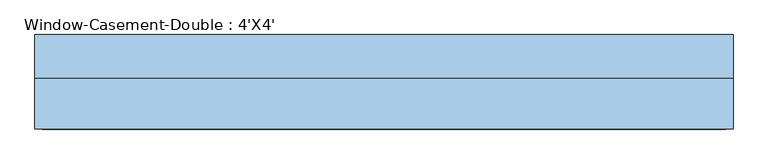
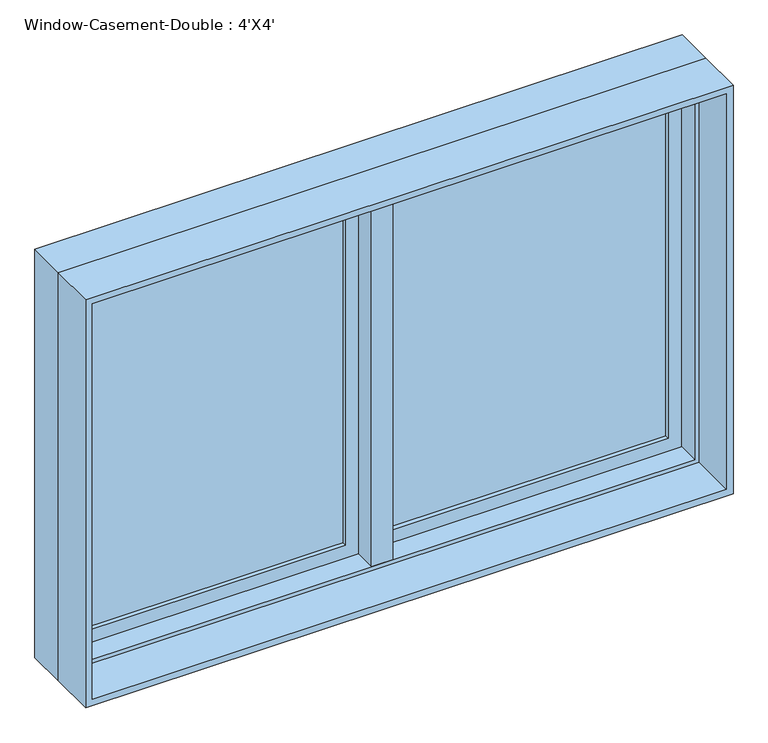
"""IFC4 building model written with IfcOpenShell, lengths in millimetres: window geometry, Window-Casement-Double : 4'X4'."""

from ifc_helpers import new_model, si_unit, frame, origin, place, context, project, spatial, polyline, outline, extrude, faceted_brep, source, transform, mapped, element, save


def window_casement_double_4_x4_bf2f09a8(model_context):
    return source(origin(), model_context, "Body", "SolidModel", [
        faceted_brep([(9.525, 133.35, 2120.9), (-9.525, 133.35, 2120.9), (-9.525, 82.55, 2120.9), (9.525, 82.55, 2120.9), (9.525, 133.35, 927.1), (9.525, 82.55, 927.1), (-9.525, 82.55, 927.1), (-9.525, 133.35, 927.1), (-9.525, 82.55, 946.15), (-9.525, 82.55, 2101.85), (-30.1625, 82.55, 946.15), (-30.1625, 82.55, 2101.85), (-30.1625, 19.05, 946.15), (-30.1625, 19.05, 2101.85), (30.1625, 19.05, 946.15), (30.1625, 19.05, 2101.85), (30.1625, 82.55, 946.15), (30.1625, 82.55, 2101.85), (9.525, 82.55, 946.15), (9.525, 82.55, 2101.85)], [[[0, 1, 2, 3]], [[4, 5, 6, 7]], [[1, 0, 4, 7]], [[2, 1, 7, 6, 8, 9]], [[9, 8, 10, 11]], [[11, 10, 12, 13]], [[13, 12, 14, 15]], [[15, 14, 16, 17]], [[17, 16, 18, 19]], [[0, 3, 19, 18, 5, 4]], [[18, 8, 6, 5]], [[9, 19, 3, 2]], [[8, 18, 16, 14, 12, 10]], [[19, 9, 11, 13, 15, 17]]]),
        extrude(outline(polyline([(-66.675, 114.3), (-66.675, 107.95), (-844.55, 107.95), (-844.55, 114.3), (-66.675, 114.3)])), frame((0.0, 0.0, 984.25), z_axis=(0.0, 0.0, 1.0), x_axis=(1.0, 0.0, 0.0)), (0.0, 0.0, 1.0), 1079.5),
        extrude(outline(polyline([(-844.55, 95.25), (-844.55, 101.6), (-66.675, 101.6), (-66.675, 95.25), (-844.55, 95.25)])), frame((0.0, 0.0, 984.25), z_axis=(0.0, 0.0, 1.0), x_axis=(1.0, 0.0, 0.0)), (0.0, 0.0, 1.0), 1079.5),
        extrude(outline(polyline([(844.55, 114.3), (844.55, 107.95), (66.675, 107.95), (66.675, 114.3), (844.55, 114.3)])), frame((0.0, 0.0, 984.25), z_axis=(0.0, 0.0, 1.0), x_axis=(1.0, 0.0, 0.0)), (0.0, 0.0, 1.0), 1079.5),
        extrude(outline(polyline([(66.675, 95.25), (66.675, 101.6), (844.55, 101.6), (844.55, 95.25), (66.675, 95.25)])), frame((0.0, 0.0, 984.25), z_axis=(0.0, 0.0, 1.0), x_axis=(1.0, 0.0, 0.0)), (0.0, 0.0, 1.0), 1079.5),
        extrude(outline(polyline([(2120.9, -901.7), (927.1, -901.7), (927.1, -9.525), (2120.9, -9.525), (2120.9, -901.7)]), holes=[polyline([(2063.75, -66.675), (984.25, -66.675), (984.25, -844.55), (2063.75, -844.55), (2063.75, -66.675)])]), frame((0.0, 82.55, 0.0), z_axis=(0.0, 1.0, 0.0), x_axis=(0.0, 0.0, 1.0)), (0.0, 0.0, 1.0), 44.45),
        extrude(outline(polyline([(927.1, 901.7), (2120.9, 901.7), (2120.9, 9.525), (927.1, 9.525), (927.1, 901.7)]), holes=[polyline([(984.25, 66.675), (2063.75, 66.675), (2063.75, 844.55), (984.25, 844.55), (984.25, 66.675)])]), frame((0.0, 82.55, 0.0), z_axis=(0.0, 1.0, 0.0), x_axis=(0.0, 0.0, 1.0)), (0.0, 0.0, 1.0), 44.45),
        extrude(outline(polyline([(2133.6, -914.4), (914.4, -914.4), (914.4, 914.4), (2133.6, 914.4), (2133.6, -914.4)]), holes=[polyline([(2114.55, 895.35), (933.45, 895.35), (933.45, -895.35), (2114.55, -895.35), (2114.55, 895.35)])]), frame((0.0, -114.3, 0.0), z_axis=(0.0, 1.0, 0.0), x_axis=(0.0, 0.0, 1.0)), (0.0, 0.0, 1.0), 133.35),
        faceted_brep([(882.65, 82.55, 2101.85), (882.65, 19.05, 2101.85), (-882.65, 19.05, 2101.85), (-882.65, 82.55, 2101.85), (901.7, 133.35, 2120.9), (901.7, 82.55, 2120.9), (-901.7, 82.55, 2120.9), (-901.7, 133.35, 2120.9), (914.4, 19.05, 2133.6), (914.4, 133.35, 2133.6), (-914.4, 133.35, 2133.6), (-914.4, 19.05, 2133.6), (-882.65, 19.05, 946.15), (-882.65, 82.55, 946.15), (-901.7, 82.55, 927.1), (-901.7, 133.35, 927.1), (-914.4, 133.35, 914.4), (-914.4, 19.05, 914.4), (882.65, 19.05, 946.15), (882.65, 82.55, 946.15), (901.7, 82.55, 927.1), (901.7, 133.35, 927.1), (914.4, 133.35, 914.4), (914.4, 19.05, 914.4)], [[[0, 1, 2, 3]], [[4, 5, 6, 7]], [[8, 9, 10, 11]], [[3, 2, 12, 13]], [[7, 6, 14, 15]], [[11, 10, 16, 17]], [[13, 12, 18, 19]], [[15, 14, 20, 21]], [[17, 16, 22, 23]], [[11, 17, 23, 8], [1, 18, 12, 2]], [[19, 18, 1, 0]], [[5, 20, 14, 6], [3, 13, 19, 0]], [[21, 20, 5, 4]], [[23, 22, 9, 8]], [[9, 22, 16, 10], [7, 15, 21, 4]]]),
    ])


if __name__ == "__main__":
    model = new_model("IFC4")
    model_context = context("Model", 3, world=origin())
    ifc_project = project(units=[si_unit("LENGTHUNIT", "METRE", prefix="MILLI")], contexts=[model_context])
    site = spatial("IfcSite", under=ifc_project)
    building = spatial("IfcBuilding", under=site)
    placement = place(None, origin())
    window_casement_double_4_x4_shape = window_casement_double_4_x4_bf2f09a8(model_context)
    element("IfcWindow", 1, ObjectType="Window-Casement-Double : 4'X4'", at=placement, inside=building, context=model_context, shape_type="MappedRepresentation", body=[
        mapped(window_casement_double_4_x4_shape, transform((0.0, 0.0, 0.0), x_axis=(1.0, 0.0, 0.0), y_axis=(0.0, 1.0, 0.0), z_axis=(0.0, 0.0, 1.0))),
    ])
    save(model, "model.ifc")

# Revit data of these elements
# Type "Window-Casement-Double : 4'X4'"
#   Type Mark = "19"
#   Fire Rating = "0.5h"
#   Assembly Code = "B2020100"
#   Analytic Construction = "Double glazing - domestic"
#   Frame Extension [instance default] = 0' - 0 1/4"
#   Window Inset [instance default] = 0' - 0"
#   Wall Thickness [instance default] = 0' - 6"
#   Interior Wall Closure [instance default] = 0' - 2 1/4"
#   Half Width = 3' - 0"
#   Visual Light Transmittance = 0.81
#   Thermal Resistance (R) = 1.8146 (h·ft²·°F)/BTU
#   Solar Heat Gain Coefficient = 0.76
#   Rough Width = 6' - 0 1/2"
#   Rough Height = 4' - 0 1/2"
#   Height = 4' - 0"
#   Heat Transfer Coefficient (U) = 0.5511 BTU/(h·ft²·°F)
#   Exterior Wall Closure [instance default] = 0' - 1 1/4"
#   Extension Jamb [instance default] = 0' - 2 1/4"
#   Default Sill Height = 3' - 0"
#   Width = 6' - 0"
#   Muntin Visibility = yes
#   Interior Trim Visibility [instance default] = yes
#   Exterior Trim Visibility [instance default] = yes
#   Extension Jamb Visibility [instance default] = yes
#   Interior Trim Material = Wood - Stained
#   Muntin Pattern = Muntin Pattern_2x2 : Muntin Pattern_2x2
#   Interior Trim = Trim-Window-Interior-Flat : Picture Frame
#   Interior Frame Material = Wood - Stained
#   Glass Panel Material = Glass
#   Exterior Trim Material = Clad - White
#   Exterior Trim = Trim-Window-Exterior-Flat : with Sill
#   Exterior Frame Material = Clad - White
#   Wall Closure = (empty or 0)
# Element 1 (IfcWindow, "Window-Casement-Double : 4'X4'")
#   Wall Thickness = 0' - 9"
#   Extension Jamb = 0' - 5 1/4"
#   Materials on its faces: "Wood - Stained", "Glass", "Clad - White"
# Materials
#   "Wood - Stained": class "Wood", colour RGB 224 178 126, transparency 0, Cost = 0
#   "Glass": class "Glass", colour RGB 0 128 192, transparency 0.75, Description = "Soda Lime Glass", Cost = 0
#   "Clad - White": class "Wood", colour RGB 242 242 238, transparency 0, Cost = 0
